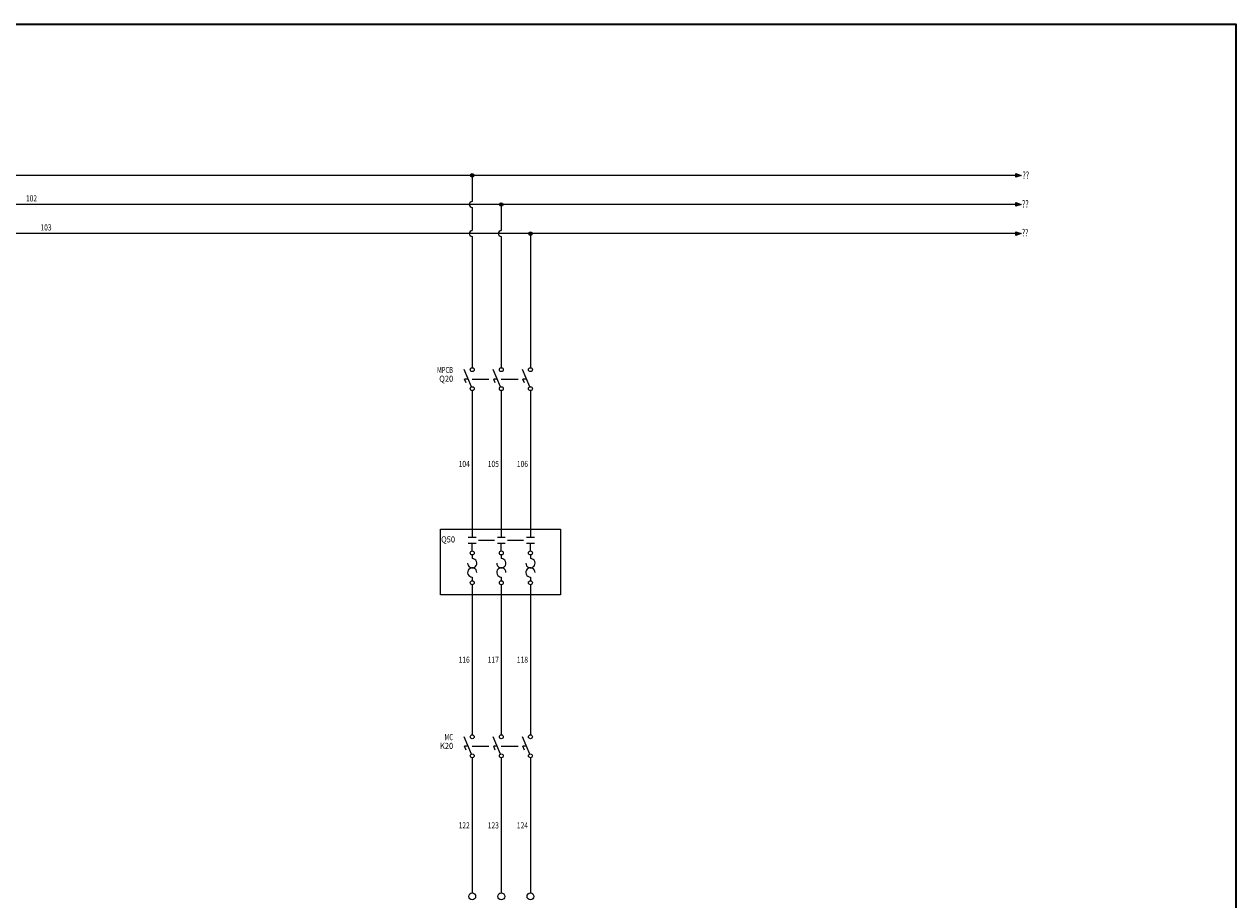
# Model space of a CAD drawing. Units: inches. Extents: x 12.5 to 62, y 4.7 to 37.4.
# Tile 5 of 5: x 37.3 to 62, y 19.5 to 37.4. Entities that reach past the tile are written whole.
import ezdxf
from ezdxf.enums import TextEntityAlignment as Align

# ---------------------------------------------------------------- set-up
doc = ezdxf.new("R2010")
doc.units = ezdxf.units.IN
doc.header["$MEASUREMENT"] = 0
for name, color, linetype, lineweight in [('16AWG-BLU', 182, 'Continuous', 25), ('16AWG-GRNYEL', 60, 'Continuous', 25), ('16AWG-RED', 1, 'Continuous', 25), ('E-ANNO-TTLB', 7, 'Continuous', 35), ('LINK', 9, 'Continuous', 13), ('LOCBOX', 7, 'Continuous', 18), ('SYMS', 7, 'Continuous', 25), ('WIRENO', 72, 'Continuous', 18), ('XREF', 7, 'Continuous', 18)]:
    doc.layers.add(name, color=color, linetype=linetype, lineweight=lineweight)
doc.layers.add('LOC', color=8, linetype='Continuous')
doc.layers.add('TAGS', color=150, linetype='Continuous')
doc.styles.add('WD', font='romans.shx')

# ---------------------------------------------------------------- blocks, each defined once
blk = doc.blocks.new('WDDOT')
for radius in [0.03, 0.0187, 0.00929]:
    blk.add_circle((0, 0), radius)
blk = doc.blocks.new('HA1S1')
for points in [[(0, 0), (0, 0.031), (0.094, 0), (0, -0.031), (0, 0)], [(0.011, 0.016), (0.011, -0.016), (0.058, 0), (0.011, 0.016)]]:
    blk.add_lwpolyline(points)
at = {"style": 'WD', "width": 0.8, "flags": 8}
blk.add_attdef('WIRENO', (0, 0.087), '', height=0.125, dxfattribs=at)
at = {"style": 'WD', "flags": 1}
for tag, p in [('SIGCODE', (-0.02, 0.047)), ('X4TERM01', (0, 0))]:
    blk.add_attdef(tag, p, '', height=0.01, dxfattribs=at)
at = {"style": 'WD', "width": 0.7}
for tag, p in [('XREF', (0, -0.181)), ('DESC1', (0, -0.356))]:
    blk.add_attdef(tag, p, '', height=0.125, dxfattribs=at)
blk = doc.blocks.new('VDS11')
for p, q in [((-0.016, -0.157), (-0.163, 0.195)), ((-0.081, 0), (-0.156, 0)), ((-0.124, -0.078), (-0.156, 0))]:
    blk.add_line(p, q)
for centre in [(0, 0.194), (0, -0.194)]:
    blk.add_circle(centre, 0.0403)
at = {"style": 'WD'}
for tag, height, flags, p in [('TERM01', 0.125, 8, (-0.069, 0.258)), ('CONTACT', 0.0125, 9, (-0.083, -0.067)), ('FAMILY', 0.0125, 9, (-0.1, -0.046)), ('MFG', 0.0125, 9, (-0.1, -0.11)), ('CAT', 0.0125, 9, (-0.1, -0.091))]:
    blk.add_attdef(tag, text='', height=height, dxfattribs=dict(at, flags=flags)).set_placement(p, align=Align.RIGHT)
for tag, width, p in [('INST', 0.7, (-0.391, 0.312)), ('LOC', 0.7, (-0.391, 0.125)), ('TAG1', 0.9, (-0.388, -0.054)), ('RATING1', 0.7, (-0.388, -0.234)), ('DESC2', 0.7, (-0.388, -0.609)), ('DESC1', 0.7, (-0.387, -0.422))]:
    blk.add_attdef(tag, text='', height=0.125, dxfattribs=dict(at, width=width)).set_placement(p, align=Align.RIGHT)
at = {"style": 'WD', "flags": 1}
for tag, p in [('X2TERM01', (0, 0.234)), ('X8TERM02', (0, -0.234))]:
    blk.add_attdef(tag, p, '', height=0.0125, dxfattribs=at)
at = {"style": 'WD'}
for tag, p in [('X4LINK', (-0.254, 0)), ('X1LINK', (0, 0))]:
    blk.add_attdef(tag, p, '', height=0.0125, dxfattribs=at)
at = {"style": 'WD', "width": 0.7}
blk.add_attdef('XREF', (0.161, -0.047), '', height=0.125, dxfattribs=at)
at = {"style": 'WD', "flags": 9}
blk.add_attdef('ASSYCODE', text='', height=0.0125, dxfattribs=at).set_placement((-0.115, -0.137), align=Align.CENTER)
at = {"style": 'WD', "flags": 8}
blk.add_attdef('TERM02', text='', height=0.125, dxfattribs=at).set_placement((-0.051, -0.267), align=Align.TOP_RIGHT)
blk = doc.blocks.new('VDS21')
for p, q in [((-0.016, -0.157), (-0.163, 0.195)), ((-0.081, 0), (-0.156, 0)), ((-0.124, -0.078), (-0.156, 0))]:
    blk.add_line(p, q)
for centre in [(0, 0.194), (0, -0.194)]:
    blk.add_circle(centre, 0.0403)
at = {"style": 'WD'}
for tag, width, p in [('INST', 0.7, (-0.373, 0.406)), ('LOC', 0.7, (-0.373, 0.221)), ('TAG2', 0.9, (-0.373, 0.031)), ('DESC1', 0.7, (-0.37, -0.344)), ('XREF', 0.7, (-0.37, -0.155)), ('DESC2', 0.7, (-0.37, -0.531))]:
    blk.add_attdef(tag, text='', height=0.125, dxfattribs=dict(at, width=width)).set_placement(p, align=Align.RIGHT)
for tag, height, flags, p in [('TERM01', 0.125, 8, (-0.069, 0.258)), ('CONTACT', 0.0125, 9, (-0.083, -0.106)), ('FAMILY', 0.0125, 9, (-0.1, -0.046))]:
    blk.add_attdef(tag, text='', height=height, dxfattribs=dict(at, flags=flags)).set_placement(p, align=Align.RIGHT)
at = {"style": 'WD', "flags": 1}
for tag, p in [('X2TERM01', (0, 0.234)), ('X8TERM02', (0, -0.234))]:
    blk.add_attdef(tag, p, '', height=0.0125, dxfattribs=at)
at = {"style": 'WD'}
for tag, p in [('X4LINK', (-0.254, 0)), ('X1LINK', (0, 0))]:
    blk.add_attdef(tag, p, '', height=0.0125, dxfattribs=at)
at = {"style": 'WD', "flags": 8}
blk.add_attdef('TERM02', text='', height=0.125, dxfattribs=at).set_placement((-0.051, -0.267), align=Align.TOP_RIGHT)
blk = doc.blocks.new('VMS21OL')
for p, q in [((-0.08, 0.062), (0.08, 0.062)), ((-0.08, -0.062), (0.08, -0.062)), ((0, -0.219), (0, -0.062)), ((0, -0.299), (0, -0.375)), ((0, -0.75), (0, -0.826))]:
    blk.add_line(p, q)
for centre in [(0, -0.259), (0, -0.866)]:
    blk.add_circle(centre, 0.04)
for centre, start, end in [((0, -0.469), 180.001, 90.002), ((0, -0.656), 0, 270.001)]:
    blk.add_arc(centre, 0.0938, start, end)
at = {"style": 'WD'}
for tag, width, p in [('INST', 0.7, (-0.352, 0.312)), ('LOC', 0.7, (-0.352, 0.125)), ('TAG2', 0.9, (-0.35, -0.045)), ('XREF', 0.7, (-0.348, -0.219)), ('DESC1', 0.7, (-0.348, -0.406)), ('DESC2', 0.7, (-0.348, -0.594)), ('DESC3', 0.7, (-0.348, -0.781))]:
    blk.add_attdef(tag, text='', height=0.125, dxfattribs=dict(at, width=width)).set_placement(p, align=Align.RIGHT)
at = {"style": 'WD', "width": 0.9, "flags": 8}
blk.add_attdef('TERM01', text='', height=0.125, dxfattribs=at).set_placement((-0.031, 0.125), align=Align.RIGHT)
at = {"style": 'WD'}
for tag, p, height, flags in [('FAMILY', (-0.181, 0.003), 0.01, 9), ('X2TERM01', (0, 0.062), 0.0125, 1), ('CONTACT', (-0.181, -0.014), 0.01, 1), ('X8TERM02', (0, -0.906), 0.0125, 1)]:
    blk.add_attdef(tag, p, '', height=height, dxfattribs=dict(at, flags=flags))
for tag, p in [('X4LINK', (-0.141, 0)), ('X1LINK', (0.125, 0))]:
    blk.add_attdef(tag, p, '', height=0.01, dxfattribs=at)
at = {"style": 'WD', "width": 0.9, "flags": 8}
blk.add_attdef('TERM02', text='', height=0.125, dxfattribs=at).set_placement((-0.031, -0.969), align=Align.TOP_RIGHT)
blk = doc.blocks.new('VT0_02')
blk.add_circle((0, 0), 0.0699)
at = {"style": 'WD', "flags": 1}
for tag, p in [('X4TERM01', (-0.07, 0)), ('X2TERM01', (0, 0.07)), ('X1TERM01', (0.07, 0)), ('X8TERM01', (0, -0.07))]:
    blk.add_attdef(tag, p, '', height=0.01, dxfattribs=at)
blk = doc.blocks.new('WD_WNH')
at = {"style": 'WD', "width": 0.8}
blk.add_attdef('WIRENO', text='', height=0.125, dxfattribs=at).set_placement((0, 0.062), align=Align.CENTER)
at = {"style": 'WD', "flags": 1}
for tag, p in [('W01USER', (0, 0.078)), ('W02USER', (0, 0.07)), ('W03USER', (0, 0.062)), ('W04USER', (0, 0.055)), ('W05USER', (0, 0.047)), ('W06USER', (0, 0.039)), ('W07USER', (0, 0.031)), ('W08USER', (0, 0.023)), ('W09USER', (0, 0.016)), ('W10USER', (0, 0.008))]:
    blk.add_attdef(tag, text='', height=0.005, dxfattribs=at).set_placement(p, align=Align.CENTER)
blk = doc.blocks.new('WD_WNV')
at = {"style": 'WD', "width": 0.8}
blk.add_attdef('WIRENO', text='', height=0.125, dxfattribs=at).set_placement((-0.05, 0), align=Align.MIDDLE_RIGHT)
at = {"style": 'WD', "flags": 1}
for tag, p in [('W01USER', (-0.062, 0.094)), ('W02USER', (-0.062, 0.086)), ('W03USER', (-0.062, 0.078)), ('W04USER', (-0.062, 0.07)), ('W05USER', (-0.062, 0.062)), ('W06USER', (-0.062, 0.055)), ('W07USER', (-0.062, 0.047)), ('W08USER', (-0.062, 0.039)), ('W09USER', (-0.062, 0.031)), ('W10USER', (-0.062, 0.023))]:
    blk.add_attdef(tag, text='', height=0.005, dxfattribs=at).set_placement(p, align=Align.CENTER)

msp = doc.modelspace()

# ---------------------------------------------------------------- linework, layer by layer
at = {"layer": '16AWG-BLU'}
for p, q in [((57.548, 33.109), (18.014, 33.109)), ((47.656, 33.109), (47.656, 30.376)), ((47.656, 29.907), (47.656, 26.92)), ((47.656, 25.951), (47.656, 22.89)), ((47.656, 22.421), (47.656, 19.667))]:
    msp.add_line(p, q, dxfattribs=at)
at = {"layer": '16AWG-GRNYEL'}
for p, q in [((57.548, 33.703), (17.421, 33.703)), ((47.062, 33.703), (47.062, 33.169)), ((47.062, 33.05), (47.062, 30.376)), ((47.062, 29.907), (47.062, 26.92)), ((47.062, 25.951), (47.062, 22.89)), ((47.062, 22.421), (47.062, 19.667))]:
    msp.add_line(p, q, dxfattribs=at)
msp.add_arc((47.062, 33.109), 0.0593, 90, 270, dxfattribs=at)
at = {"layer": '16AWG-RED'}
for p, q in [((57.544, 34.296), (16.828, 34.296)), ((46.469, 34.296), (46.469, 33.762)), ((46.469, 33.643), (46.469, 33.169)), ((46.469, 33.05), (46.469, 30.376)), ((46.469, 29.907), (46.469, 26.92)), ((46.469, 25.951), (46.469, 22.89)), ((46.469, 22.421), (46.469, 19.667))]:
    msp.add_line(p, q, dxfattribs=at)
for centre in [(46.469, 33.703), (46.469, 33.109)]:
    msp.add_arc(centre, 0.0593, 90, 270, dxfattribs=at)
at = {"layer": 'E-ANNO-TTLB'}
msp.add_lwpolyline([(12.524, 37.377), (62.033, 37.377), (62.033, 4.741), (12.524, 4.741)], close=True, dxfattribs=at)
at = {"layer": 'LINK'}
for points in [[(46.469, 30.141), (46.808, 30.141)], [(47.062, 30.141), (47.402, 30.141)], [(46.594, 26.857), (46.922, 26.857)], [(47.187, 26.857), (47.515, 26.857)], [(46.469, 22.656), (46.808, 22.656)], [(47.062, 22.656), (47.402, 22.656)]]:
    msp.add_lwpolyline(points, dxfattribs=at)
at = {"layer": 'LOCBOX'}
msp.add_lwpolyline([(45.821, 27.08), (48.27, 27.08), (48.27, 25.744), (45.821, 25.744)], close=True, dxfattribs=at)

# ---------------------------------------------------------------- block references
at = {"layer": 'SYMS', "xscale": 1.186465831832244, "yscale": 1.186465831832244, "zscale": 1.186465831832244}
for p in [(46.469, 34.296), (47.062, 33.703), (47.656, 33.109)]:
    msp.add_blockref('WDDOT', p, dxfattribs=at)
at = {"layer": 'SYMS'}
ref = msp.add_blockref('HA1S1', (57.548, 34.296), dxfattribs=dict(at, xscale=1.186465831832244, yscale=1.186465831832244, zscale=1.186465831832244))
ref.add_attrib('XREF', '??', (57.685, 34.224), dxfattribs={"layer": 'XREF', "height": 0.1483, "style": 'WD', "width": 0.7})
ref = msp.add_blockref('HA1S1', (57.548, 33.703), dxfattribs=dict(at, xscale=1.186465831832244, yscale=1.186465831832244, zscale=1.186465831832244))
ref.add_attrib('XREF', '??', (57.676, 33.64), dxfattribs={"layer": 'XREF', "height": 0.1483, "style": 'WD', "width": 0.7})
ref = msp.add_blockref('HA1S1', (57.548, 33.109), dxfattribs=dict(at, xscale=1.186465831832244, yscale=1.186465831832244, zscale=1.186465831832244))
ref.add_attrib('XREF', '??', (57.671, 33.053), dxfattribs={"layer": 'XREF', "height": 0.1483, "style": 'WD', "width": 0.7})
ref = msp.add_blockref('VDS11', (46.469, 30.141), dxfattribs=at)
ref.add_attrib('TAG1', 'Q20', dxfattribs={"layer": 'TAGS', "height": 0.125, "style": 'WD', "width": 0.9}).set_placement((46.081, 30.087), align=Align.RIGHT)
ref.add_attrib('LOC', 'MPCB', dxfattribs={"layer": 'LOC', "height": 0.125, "style": 'WD', "width": 0.7}).set_placement((46.078, 30.266), align=Align.RIGHT)
for name, p in [('VDS21', (47.062, 30.141)), ('VDS21', (47.656, 30.141)), ('VMS21OL', (47.062, 26.857)), ('VMS21OL', (47.656, 26.857)), ('VDS21', (47.062, 22.656)), ('VDS21', (47.656, 22.656)), ('VT0_02', (46.469, 19.597)), ('VT0_02', (47.062, 19.597)), ('VT0_02', (47.656, 19.597))]:
    msp.add_blockref(name, p, dxfattribs=at)
ref = msp.add_blockref('VMS21OL', (46.469, 26.857), dxfattribs=at)
ref.add_attrib('TAG2', 'Q50', dxfattribs={"layer": 'TAGS', "height": 0.125, "style": 'WD', "width": 0.9}).set_placement((46.119, 26.812), align=Align.RIGHT)
ref = msp.add_blockref('VDS11', (46.469, 22.656), dxfattribs=at)
ref.add_attrib('TAG1', 'K20', dxfattribs={"layer": 'TAGS', "height": 0.125, "style": 'WD', "width": 0.9}).set_placement((46.081, 22.602), align=Align.RIGHT)
ref.add_attrib('LOC', 'MC', dxfattribs={"layer": 'LOC', "height": 0.125, "style": 'WD', "width": 0.7}).set_placement((46.078, 22.781), align=Align.RIGHT)
at = {"layer": 'WIRENO'}
ref = msp.add_blockref('WD_WNH', (37.485, 33.703), dxfattribs=at)
ref.add_attrib('WIRENO', '102', dxfattribs={"linetype": 'Continuous', "height": 0.125, "style": 'WD', "width": 0.8}).set_placement((37.485, 33.765), align=Align.CENTER)
ref = msp.add_blockref('WD_WNH', (37.781, 33.109), dxfattribs=at)
ref.add_attrib('WIRENO', '103', dxfattribs={"linetype": 'Continuous', "height": 0.125, "style": 'WD', "width": 0.8}).set_placement((37.781, 33.172), align=Align.CENTER)
ref = msp.add_blockref('WD_WNV', (46.469, 28.413), dxfattribs=at)
ref.add_attrib('WIRENO', '104', dxfattribs={"linetype": 'Continuous', "height": 0.125, "style": 'WD', "width": 0.8}).set_placement((46.419, 28.413), align=Align.MIDDLE_RIGHT)
ref = msp.add_blockref('WD_WNV', (47.062, 28.413), dxfattribs=at)
ref.add_attrib('WIRENO', '105', dxfattribs={"linetype": 'Continuous', "height": 0.125, "style": 'WD', "width": 0.8}).set_placement((47.012, 28.413), align=Align.MIDDLE_RIGHT)
ref = msp.add_blockref('WD_WNV', (47.656, 28.413), dxfattribs=at)
ref.add_attrib('WIRENO', '106', dxfattribs={"linetype": 'Continuous', "height": 0.125, "style": 'WD', "width": 0.8}).set_placement((47.606, 28.413), align=Align.MIDDLE_RIGHT)
ref = msp.add_blockref('WD_WNV', (46.469, 24.421), dxfattribs=at)
ref.add_attrib('WIRENO', '116', dxfattribs={"linetype": 'Continuous', "height": 0.125, "style": 'WD', "width": 0.8}).set_placement((46.419, 24.421), align=Align.MIDDLE_RIGHT)
ref = msp.add_blockref('WD_WNV', (47.062, 24.421), dxfattribs=at)
ref.add_attrib('WIRENO', '117', dxfattribs={"linetype": 'Continuous', "height": 0.125, "style": 'WD', "width": 0.8}).set_placement((47.012, 24.421), align=Align.MIDDLE_RIGHT)
ref = msp.add_blockref('WD_WNV', (47.656, 24.421), dxfattribs=at)
ref.add_attrib('WIRENO', '118', dxfattribs={"linetype": 'Continuous', "height": 0.125, "style": 'WD', "width": 0.8}).set_placement((47.606, 24.421), align=Align.MIDDLE_RIGHT)
ref = msp.add_blockref('WD_WNV', (46.469, 21.044), dxfattribs=at)
ref.add_attrib('WIRENO', '122', dxfattribs={"linetype": 'Continuous', "height": 0.125, "style": 'WD', "width": 0.8}).set_placement((46.419, 21.044), align=Align.MIDDLE_RIGHT)
ref = msp.add_blockref('WD_WNV', (47.062, 21.044), dxfattribs=at)
ref.add_attrib('WIRENO', '123', dxfattribs={"linetype": 'Continuous', "height": 0.125, "style": 'WD', "width": 0.8}).set_placement((47.012, 21.044), align=Align.MIDDLE_RIGHT)
ref = msp.add_blockref('WD_WNV', (47.656, 21.044), dxfattribs=at)
ref.add_attrib('WIRENO', '124', dxfattribs={"linetype": 'Continuous', "height": 0.125, "style": 'WD', "width": 0.8}).set_placement((47.606, 21.044), align=Align.MIDDLE_RIGHT)

doc.saveas('drawing.dxf')
